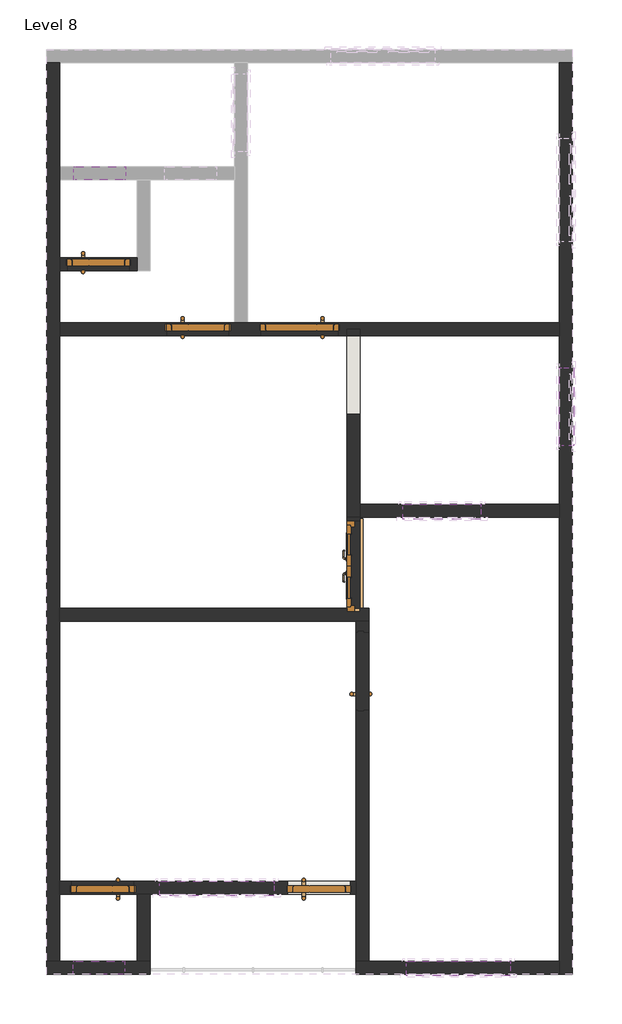
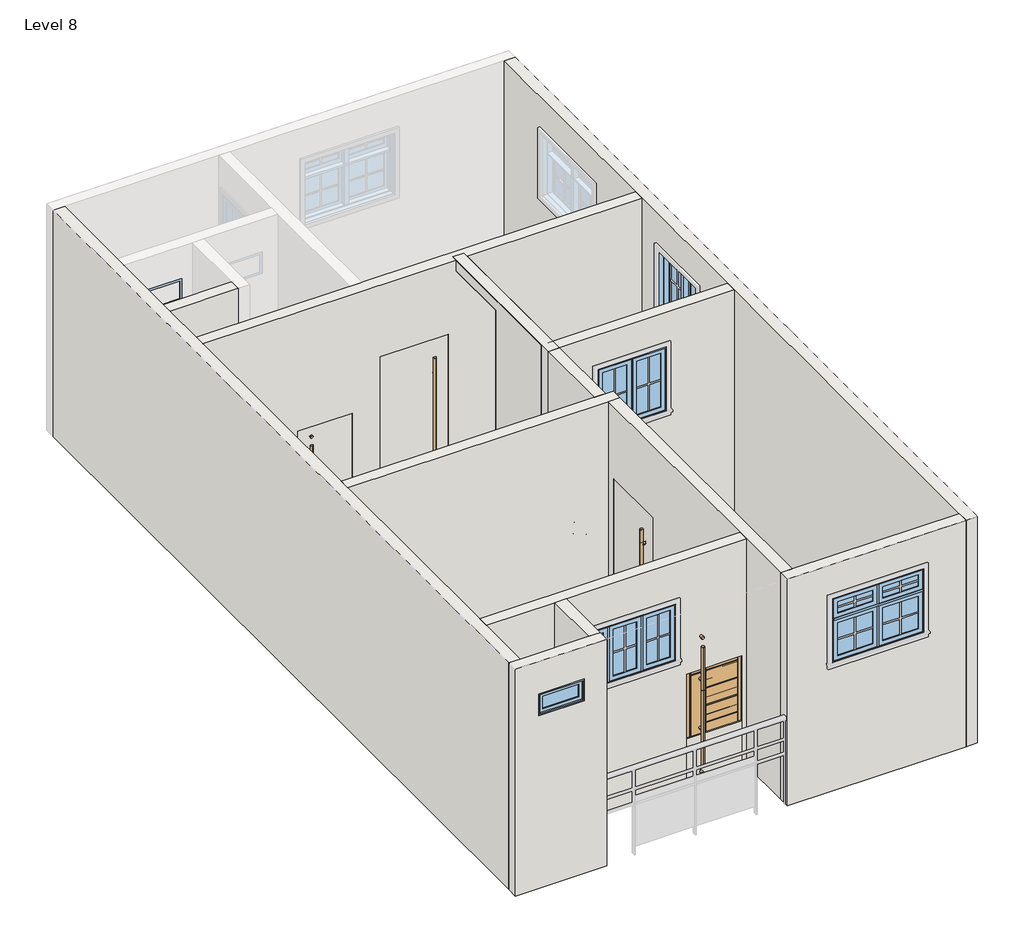
# One storey, part 1 of 2: 22 walls, 8 doors, 8 windows.
"""IFC4 building model written with IfcOpenShell, lengths in millimetres."""

from ifc_helpers import new_model, si_unit, frame, origin, place, context, project, spatial, polyline, outline, extrude, faceted_brep, transform, mapped, element, save
from components import door_9b787682, door_dc81b0c5, door_3_5c4206ef, door_3_79df91aa, door_2576ec39, door_55c03dfd, fixed_2_65c13adb, window_61697a4f, m_window_casement_double_3_e0bd8fa3, m_window_casement_double_awning_double_4_7efa9bbd

model = new_model("IFC4")

# Units and contexts
model_context = context("Model", 3, world=origin())
ifc_project = project(units=[si_unit("LENGTHUNIT", "METRE", prefix="MILLI")], contexts=[model_context])

# Site, building, storey
site = spatial("IfcSite", under=ifc_project)
building = spatial("IfcBuilding", under=site)
storey = spatial("IfcBuildingStorey", under=building, Name="Level 8", Elevation=13411.2)

# Doors
placement = place(None, origin())
door_shape = door_9b787682(model_context)
element("IfcDoor", 1, ObjectType="2'5\"", at=placement, inside=storey, context=model_context, shape_type="MappedRepresentation", body=[
    mapped(door_shape, transform((-22033.2963079, 3049.4742053, 13411.2), x_axis=(1.0, 0.0, 0.0), y_axis=(0.0, 1.0, 0.0), z_axis=(0.0, 0.0, 1.0))),
])
element("IfcDoor", 2, ObjectType="2'5\"", at=placement, inside=storey, context=model_context, shape_type="MappedRepresentation", body=[
    mapped(door_shape, transform((-23201.6963079, 3811.4742053, 13411.2), x_axis=(1.0, 0.0, 0.0), y_axis=(0.0, 1.0, 0.0), z_axis=(0.0, 0.0, 1.0))),
])
element("IfcDoor", 3, ObjectType="2'5\"", at=placement, inside=storey, context=model_context, shape_type="MappedRepresentation", body=[
    mapped(door_shape, transform((-23150.8963079, -3503.7257947, 13411.2), x_axis=(-1.0, 0.0, 0.0), y_axis=(0.0, -1.0, 0.0), z_axis=(0.0, 0.0, 1.0))),
])
door_2_shape = door_dc81b0c5(model_context)
element("IfcDoor", 4, ObjectType="2'5\"", at=placement, inside=storey, context=model_context, shape_type="MappedRepresentation", body=[
    mapped(door_2_shape, transform((-20610.8963079, -3503.7257947, 13457.4445349), x_axis=(1.0, 0.0, 0.0), y_axis=(0.0, 1.0, 0.0), z_axis=(0.0, 0.0, 1.0))),
])
element("IfcDoor", 5, ObjectType="2'5\"", at=placement, inside=storey, context=model_context, shape_type="MappedRepresentation", body=[
    mapped(door_2_shape, transform((-20610.8963079, -3503.7257947, 14067.0445349), x_axis=(1.0, 0.0, 0.0), y_axis=(0.0, 1.0, 0.0), z_axis=(0.0, 0.0, 1.0))),
])
door_3_shape = door_3_5c4206ef(model_context)
element("IfcDoor", 6, ObjectType="3'", at=placement, inside=storey, context=model_context, shape_type="MappedRepresentation", body=[
    mapped(door_3_shape, transform((-20102.8963079, -963.7257947, 13411.2), x_axis=(0.0, 1.0, 0.0), y_axis=(-1.0, 0.0, 0.0), z_axis=(0.0, 0.0, 1.0))),
])
door_3_2_shape = door_3_79df91aa(model_context)
element("IfcDoor", 7, ObjectType="3'", at=placement, inside=storey, context=model_context, shape_type="MappedRepresentation", body=[
    mapped(door_3_2_shape, transform((-20839.4963079, 3049.4742053, 13411.2), x_axis=(-1.0, 0.0, 0.0), y_axis=(0.0, -1.0, 0.0), z_axis=(0.0, 0.0, 1.0))),
])
door_4_shape = door_2576ec39(model_context)
door_5_shape = door_55c03dfd(model_context)
element("IfcDoor", 8, ObjectType="ExtDbl (8) : 3'6\"", at=placement, inside=storey, context=model_context, shape_type="MappedRepresentation", body=[
    mapped(door_4_shape, transform((-20204.4963079, 268.1742053, 13411.2), x_axis=(0.0, -1.0, 0.0), y_axis=(1.0, 0.0, 0.0), z_axis=(0.0, 0.0, 1.0))),
    mapped(door_5_shape, transform((-20204.4963079, 268.1742053, 13411.2), x_axis=(0.0, -1.0, 0.0), y_axis=(1.0, 0.0, 0.0), z_axis=(0.0, 0.0, 1.0))),
])

# Walls
element("IfcWall", 9, ObjectType="Generic - 6\"", at=placement, inside=storey, context=model_context, shape_type="Brep", body=[
    faceted_brep([(-17791.4963079, 6173.6742053, 13411.2), (-17791.4963079, 3125.6742053, 13411.2), (-17791.4963079, 2973.2742053, 13411.2), (-17791.4963079, 992.0742053, 13411.2), (-17791.4963079, 839.6742053, 13411.2), (-17791.4963079, -4367.3257947, 13411.2), (-17791.4963079, -4519.7257947, 13411.2), (-17791.4963079, -4519.7257947, 16611.6), (-17791.4963079, -4367.3257947, 16611.6), (-17791.4963079, 839.6742053, 16611.6), (-17791.4963079, 992.0742053, 16611.6), (-17791.4963079, 2973.2742053, 16611.6), (-17791.4963079, 3125.6742053, 16611.6), (-17791.4963079, 6173.6742053, 16611.6), (-17791.4963079, 4071.8242053, 16140.0), (-17791.4963079, 4071.8242053, 15240.0), (-17791.4963079, 5291.0242053, 15240.0), (-17791.4963079, 5291.0242053, 16140.0), (-17791.4963079, 1682.6367053, 16140.0), (-17791.4963079, 1682.6367053, 15240.0), (-17791.4963079, 2597.0367053, 15240.0), (-17791.4963079, 2597.0367053, 16140.0), (-17639.0963079, 6173.6742053, 13411.2), (-17639.0963079, 6173.6742053, 16611.6), (-17639.0963079, -4519.7257947, 16611.6), (-17639.0963079, -4519.7257947, 13411.2), (-17639.0963079, 4071.8242053, 16140.0), (-17639.0963079, 5291.0242053, 16140.0), (-17639.0963079, 5291.0242053, 15240.0), (-17639.0963079, 4071.8242053, 15240.0), (-17639.0963079, 1682.6367053, 16140.0), (-17639.0963079, 2597.0367053, 16140.0), (-17639.0963079, 2597.0367053, 15240.0), (-17639.0963079, 1682.6367053, 15240.0)], [[[0, 1, 2, 3, 4, 5, 6, 7, 8, 9, 10, 11, 12, 13], [14, 15, 16, 17], [18, 19, 20, 21]], [[22, 23, 24, 25], [26, 27, 28, 29], [30, 31, 32, 33]], [[6, 5, 4, 3, 2, 1, 0, 22, 25]], [[13, 12, 11, 10, 9, 8, 7, 24, 23]], [[0, 13, 23, 22]], [[7, 6, 25, 24]], [[15, 14, 26, 29]], [[16, 15, 29, 28]], [[17, 16, 28, 27]], [[14, 17, 27, 26]], [[19, 18, 30, 33]], [[20, 19, 33, 32]], [[21, 20, 32, 31]], [[18, 21, 31, 30]]]),
])
element("IfcWall", 10, ObjectType="Generic - 6\"", at=placement, inside=storey, context=model_context, shape_type="Brep", body=[
    faceted_brep([(-17791.4963079, -4367.3257947, 13411.2), (-20026.6963079, -4367.3257947, 13411.2), (-20179.0963079, -4367.3257947, 13411.2), (-20179.0963079, -4367.3257947, 16611.6), (-20026.6963079, -4367.3257947, 16611.6), (-17791.4963079, -4367.3257947, 16611.6), (-19585.5697454, -4367.3257947, 16140.0), (-19585.5697454, -4367.3257947, 15240.0), (-18366.3697454, -4367.3257947, 15240.0), (-18366.3697454, -4367.3257947, 16140.0), (-17791.4963079, -4519.7257947, 13411.2), (-17791.4963079, -4519.7257947, 16611.6), (-20179.0963079, -4519.7257947, 16611.6), (-20179.0963079, -4519.7257947, 13411.2), (-19585.5697454, -4519.7257947, 16140.0), (-18366.3697454, -4519.7257947, 16140.0), (-18366.3697454, -4519.7257947, 15240.0), (-19585.5697454, -4519.7257947, 15240.0)], [[[0, 1, 2, 3, 4, 5], [6, 7, 8, 9]], [[10, 11, 12, 13], [14, 15, 16, 17]], [[2, 1, 0, 10, 13]], [[5, 4, 3, 12, 11]], [[0, 5, 11, 10]], [[3, 2, 13, 12]], [[7, 6, 14, 17]], [[8, 7, 17, 16]], [[9, 8, 16, 15]], [[6, 9, 15, 14]]]),
])
element("IfcWall", 11, ObjectType="Generic - 6\"", at=placement, inside=storey, context=model_context, shape_type="Brep", body=[
    faceted_brep([(-23811.2963079, -4519.7257947, 13411.2), (-22592.0963079, -4519.7257947, 13411.2), (-22592.0963079, -4519.7257947, 16611.6), (-23811.2963079, -4519.7257947, 16611.6), (-23500.5431829, -4519.7257947, 16154.4), (-22890.9431829, -4519.7257947, 16154.4), (-22890.9431829, -4519.7257947, 15849.6), (-23500.5431829, -4519.7257947, 15849.6), (-23811.2963079, -4367.3257947, 13411.2), (-23811.2963079, -4367.3257947, 16611.6), (-23658.8963079, -4367.3257947, 16611.6), (-22744.4963079, -4367.3257947, 16611.6), (-22592.0963079, -4367.3257947, 16611.6), (-22592.0963079, -4367.3257947, 13411.2), (-22744.4963079, -4367.3257947, 13411.2), (-23658.8963079, -4367.3257947, 13411.2), (-23500.5431829, -4367.3257947, 16154.4), (-23500.5431829, -4367.3257947, 15849.6), (-22890.9431829, -4367.3257947, 15849.6), (-22890.9431829, -4367.3257947, 16154.4)], [[[0, 1, 2, 3], [4, 5, 6, 7]], [[8, 9, 10, 11, 12, 13, 14, 15], [16, 17, 18, 19]], [[1, 0, 8, 15, 14, 13]], [[3, 2, 12, 11, 10, 9]], [[0, 3, 9, 8]], [[2, 1, 13, 12]], [[17, 16, 4, 7]], [[18, 17, 7, 6]], [[19, 18, 6, 5]], [[16, 19, 5, 4]]]),
])
element("IfcWall", 12, ObjectType="Generic - 6\"", at=placement, inside=storey, context=model_context, shape_type="Brep", body=[
    faceted_brep([(-23658.8963079, -4367.3257947, 13411.2), (-23658.8963079, -3579.9257947, 13411.2), (-23658.8963079, -3427.5257947, 13411.2), (-23658.8963079, -379.5257947, 13411.2), (-23658.8963079, -227.1257947, 13411.2), (-23658.8963079, 2973.2742053, 13411.2), (-23658.8963079, 3125.6742053, 13411.2), (-23658.8963079, 3735.2742053, 13411.2), (-23658.8963079, 3887.6742053, 13411.2), (-23658.8963079, 4802.0742053, 13411.2), (-23658.8963079, 4954.4742053, 13411.2), (-23658.8963079, 6173.6742053, 13411.2), (-23658.8963079, 6173.6742053, 16611.6), (-23658.8963079, 4954.4742053, 16611.6), (-23658.8963079, 4802.0742053, 16611.6), (-23658.8963079, 3887.6742053, 16611.6), (-23658.8963079, 3735.2742053, 16611.6), (-23658.8963079, 3125.6742053, 16611.6), (-23658.8963079, 2973.2742053, 16611.6), (-23658.8963079, -227.1257947, 16611.6), (-23658.8963079, -379.5257947, 16611.6), (-23658.8963079, -3427.5257947, 16611.6), (-23658.8963079, -3579.9257947, 16611.6), (-23658.8963079, -4367.3257947, 16611.6), (-23811.2963079, -4367.3257947, 13411.2), (-23811.2963079, -4367.3257947, 16611.6), (-23811.2963079, 6173.6742053, 16611.6), (-23811.2963079, 6173.6742053, 13411.2)], [[[0, 1, 2, 3, 4, 5, 6, 7, 8, 9, 10, 11, 12, 13, 14, 15, 16, 17, 18, 19, 20, 21, 22, 23]], [[24, 25, 26, 27]], [[11, 10, 9, 8, 7, 6, 5, 4, 3, 2, 1, 0, 24, 27]], [[23, 22, 21, 20, 19, 18, 17, 16, 15, 14, 13, 12, 26, 25]], [[12, 11, 27, 26]], [[0, 23, 25, 24]]]),
])
element("IfcWall", 13, ObjectType="Generic - 6\"", at=placement, inside=storey, context=model_context, shape_type="Brep", body=[
    faceted_brep([(-17791.4963079, 2973.2742053, 16611.6), (-20128.2963079, 2973.2742053, 16611.6), (-20280.6963079, 2973.2742053, 16611.6), (-23658.8963079, 2973.2742053, 16611.6), (-23658.8963079, 2973.2742053, 13411.2), (-22401.5963079, 2973.2742053, 13411.2), (-22401.5963079, 2973.2742053, 14935.2), (-21664.9963079, 2973.2742053, 14935.2), (-21664.9963079, 2973.2742053, 13411.2), (-21296.6963079, 2973.2742053, 13411.2), (-21296.6963079, 2973.2742053, 15600.7), (-20382.2963079, 2973.2742053, 15600.7), (-20382.2963079, 2973.2742053, 13411.2), (-20280.6963079, 2973.2742053, 13411.2), (-20128.2963079, 2973.2742053, 13411.2), (-17791.4963079, 2973.2742053, 13411.2), (-23658.8963079, 3125.6742053, 16611.6), (-21601.4963079, 3125.6742053, 16611.6), (-21449.0963079, 3125.6742053, 16611.6), (-17791.4963079, 3125.6742053, 16611.6), (-17791.4963079, 3125.6742053, 13411.2), (-20382.2963079, 3125.6742053, 13411.2), (-20382.2963079, 3125.6742053, 15600.7), (-21296.6963079, 3125.6742053, 15600.7), (-21296.6963079, 3125.6742053, 13411.2), (-21449.0963079, 3125.6742053, 13411.2), (-21601.4963079, 3125.6742053, 13411.2), (-21664.9963079, 3125.6742053, 13411.2), (-21664.9963079, 3125.6742053, 14935.2), (-22401.5963079, 3125.6742053, 14935.2), (-22401.5963079, 3125.6742053, 13411.2), (-23658.8963079, 3125.6742053, 13411.2), (-22401.5963079, 3105.6742053, 13411.2), (-22416.5963079, 3105.6742053, 13411.2), (-22416.5963079, 3028.6742053, 13411.2), (-22401.5963079, 3028.6742053, 13411.2), (-20382.2963079, 3028.6742053, 13411.2), (-20367.2963079, 3028.6742053, 13411.2), (-20367.2963079, 3105.6742053, 13411.2), (-20382.2963079, 3105.6742053, 13411.2), (-21296.6963079, 3028.6742053, 13411.2), (-21664.9963079, 3028.6742053, 13411.2), (-21649.9963079, 3028.6742053, 13411.2), (-21649.9963079, 3105.6742053, 13411.2), (-21664.9963079, 3105.6742053, 13411.2), (-21296.6963079, 3105.6742053, 13411.2), (-21311.6963079, 3105.6742053, 13411.2), (-21311.6963079, 3028.6742053, 13411.2), (-21296.6963079, 3105.6742053, 15600.7), (-20382.2963079, 3105.6742053, 15600.7), (-20382.2963079, 3028.6742053, 15600.7), (-21296.6963079, 3028.6742053, 15600.7), (-21311.6963079, 3105.6742053, 15615.7), (-20367.2963079, 3105.6742053, 15615.7), (-20367.2963079, 3028.6742053, 15615.7), (-21311.6963079, 3028.6742053, 15615.7), (-21664.9963079, 3105.6742053, 14935.2), (-22401.5963079, 3105.6742053, 14935.2), (-22401.5963079, 3028.6742053, 14935.2), (-21664.9963079, 3028.6742053, 14935.2), (-22416.5963079, 3105.6742053, 14950.2), (-21649.9963079, 3105.6742053, 14950.2), (-21649.9963079, 3028.6742053, 14950.2), (-22416.5963079, 3028.6742053, 14950.2)], [[[0, 1, 2, 3, 4, 5, 6, 7, 8, 9, 10, 11, 12, 13, 14, 15]], [[16, 17, 18, 19, 20, 21, 22, 23, 24, 25, 26, 27, 28, 29, 30, 31]], [[4, 31, 30, 32, 33, 34, 35, 5]], [[20, 15, 14, 13, 12, 36, 37, 38, 39, 21]], [[40, 9, 8, 41, 42, 43, 44, 27, 26, 25, 24, 45, 46, 47]], [[3, 2, 1, 0, 19, 18, 17, 16]], [[0, 15, 20, 19]], [[4, 3, 16, 31]], [[48, 23, 22, 49]], [[50, 11, 10, 51]], [[23, 48, 45, 24]], [[51, 10, 9, 40]], [[49, 22, 21, 39]], [[11, 50, 36, 12]], [[52, 53, 54, 55]], [[52, 55, 47, 46]], [[50, 51, 40, 47, 55, 54, 37, 36]], [[54, 53, 38, 37]], [[48, 49, 39, 38, 53, 52, 46, 45]], [[28, 56, 57, 29]], [[6, 58, 59, 7]], [[56, 28, 27, 44]], [[7, 59, 41, 8]], [[29, 57, 32, 30]], [[58, 6, 5, 35]], [[60, 61, 62, 63]], [[62, 61, 43, 42]], [[59, 58, 35, 34, 63, 62, 42, 41]], [[60, 63, 34, 33]], [[57, 56, 44, 43, 61, 60, 33, 32]]]),
])
element("IfcWall", 14, ObjectType="Generic - 6\"", at=placement, inside=storey, context=model_context, shape_type="Brep", body=[
    faceted_brep([(-20280.6963079, 3049.4742053, 16611.6), (-20280.6963079, 3049.4742053, 13411.2), (-20280.6963079, 839.6742053, 13411.2), (-20280.6963079, 839.6742053, 16611.6), (-20280.6963079, 2974.7724011, 16459.2), (-20280.6963079, 2050.5574639, 16459.2), (-20280.6963079, 2050.5574639, 14020.8), (-20280.6963079, 2974.7724011, 14020.8), (-20128.2963079, 839.6742053, 13411.2), (-20128.2963079, 992.0742053, 13411.2), (-20128.2963079, 3049.4742053, 13411.2), (-20128.2963079, 3049.4742053, 16611.6), (-20128.2963079, 992.0742053, 16611.6), (-20128.2963079, 839.6742053, 16611.6), (-20128.2963079, 2050.5574639, 16459.2), (-20128.2963079, 2974.7724011, 16459.2), (-20128.2963079, 2974.7724011, 14020.8), (-20128.2963079, 2050.5574639, 14020.8)], [[[0, 1, 2, 3], [4, 5, 6, 7]], [[8, 9, 10, 11, 12, 13], [14, 15, 16, 17]], [[2, 1, 10, 9, 8]], [[0, 3, 13, 12, 11]], [[3, 2, 8, 13]], [[4, 15, 14, 5]], [[6, 17, 16, 7]], [[15, 4, 7, 16]], [[5, 14, 17, 6]], [[0, 11, 10, 1]]]),
])
element("IfcWall", 15, ObjectType="Generic - 6\"", at=placement, inside=storey, context=model_context, shape_type="SweptSolid", body=[
    extrude(outline(polyline([(13411.2, -20128.2963079), (13411.2, -17791.4963079), (16611.6, -17791.4963079), (16611.6, -20128.2963079), (13411.2, -20128.2963079)]), holes=[polyline([(16140.0, -19624.1658391), (16140.0, -18709.7658391), (15240.0, -18709.7658391), (15240.0, -19624.1658391), (16140.0, -19624.1658391)])]), frame((0.0, 839.6742053, 0.0), z_axis=(0.0, 1.0, 0.0), x_axis=(0.0, 0.0, 1.0)), (0.0, 0.0, 1.0), 152.4),
])
element("IfcWall", 16, ObjectType="Generic - 6\"", at=placement, inside=storey, context=model_context, shape_type="Brep", body=[
    faceted_brep([(-23658.8963079, -379.5257947, 13411.2), (-20179.0963079, -379.5257947, 13411.2), (-20026.6963079, -379.5257947, 13411.2), (-20026.6963079, -379.5257947, 16611.6), (-20179.0963079, -379.5257947, 16611.6), (-23658.8963079, -379.5257947, 16611.6), (-23658.8963079, -227.1257947, 16611.6), (-20280.6963079, -227.1257947, 16611.6), (-20128.2963079, -227.1257947, 16611.6), (-20026.6963079, -227.1257947, 16611.6), (-20026.6963079, -227.1257947, 13411.2), (-20128.2963079, -227.1257947, 13411.2), (-20128.2963079, -227.1257947, 15521.2), (-20280.6963079, -227.1257947, 15521.2), (-20280.6963079, -227.1257947, 13411.2), (-23658.8963079, -227.1257947, 13411.2), (-20280.6963079, -265.2257947, 13411.2), (-20128.2963079, -265.2257947, 13411.2), (-20280.6963079, -265.2257947, 15521.2), (-20128.2963079, -265.2257947, 15521.2)], [[[0, 1, 2, 3, 4, 5]], [[6, 7, 8, 9, 10, 11, 12, 13, 14, 15]], [[2, 1, 0, 15, 14, 16, 17, 11, 10]], [[5, 4, 3, 9, 8, 7, 6]], [[0, 5, 6, 15]], [[3, 2, 10, 9]], [[18, 16, 14, 13]], [[17, 19, 12, 11]], [[19, 18, 13, 12]], [[16, 18, 19, 17]]]),
])
element("IfcWall", 17, ObjectType="Generic - 6\"", at=placement, inside=storey, context=model_context, shape_type="Brep", body=[
    faceted_brep([(-20179.0963079, -4367.3257947, 16611.6), (-20179.0963079, -3579.9257947, 16611.6), (-20179.0963079, -3427.5257947, 16611.6), (-20179.0963079, -379.5257947, 16611.6), (-20179.0963079, -379.5257947, 13411.2), (-20179.0963079, -506.5257947, 13411.2), (-20179.0963079, -506.5257947, 15600.7), (-20179.0963079, -1420.9257947, 15600.7), (-20179.0963079, -1420.9257947, 13411.2), (-20179.0963079, -3427.5257947, 13411.2), (-20179.0963079, -3579.9257947, 13411.2), (-20179.0963079, -4367.3257947, 13411.2), (-20026.6963079, -379.5257947, 16611.6), (-20026.6963079, -4367.3257947, 16611.6), (-20026.6963079, -4367.3257947, 13411.2), (-20026.6963079, -1420.9257947, 13411.2), (-20026.6963079, -1420.9257947, 15600.7), (-20026.6963079, -506.5257947, 15600.7), (-20026.6963079, -506.5257947, 13411.2), (-20026.6963079, -379.5257947, 13411.2), (-20082.0963079, -506.5257947, 13411.2), (-20082.0963079, -491.5257947, 13411.2), (-20159.0963079, -491.5257947, 13411.2), (-20159.0963079, -506.5257947, 13411.2), (-20159.0963079, -1420.9257947, 13411.2), (-20159.0963079, -1435.9257947, 13411.2), (-20082.0963079, -1435.9257947, 13411.2), (-20082.0963079, -1420.9257947, 13411.2), (-20159.0963079, -506.5257947, 15600.7), (-20159.0963079, -1420.9257947, 15600.7), (-20082.0963079, -1420.9257947, 15600.7), (-20082.0963079, -506.5257947, 15600.7), (-20159.0963079, -1435.9257947, 15615.7), (-20159.0963079, -491.5257947, 15615.7), (-20082.0963079, -491.5257947, 15615.7), (-20082.0963079, -1435.9257947, 15615.7)], [[[0, 1, 2, 3, 4, 5, 6, 7, 8, 9, 10, 11]], [[12, 13, 14, 15, 16, 17, 18, 19]], [[4, 19, 18, 20, 21, 22, 23, 5]], [[14, 11, 10, 9, 8, 24, 25, 26, 27, 15]], [[3, 2, 1, 0, 13, 12]], [[0, 11, 14, 13]], [[4, 3, 12, 19]], [[6, 28, 29, 7]], [[16, 30, 31, 17]], [[28, 6, 5, 23]], [[17, 31, 20, 18]], [[7, 29, 24, 8]], [[30, 16, 15, 27]], [[32, 33, 34, 35]], [[34, 33, 22, 21]], [[31, 30, 27, 26, 35, 34, 21, 20]], [[32, 35, 26, 25]], [[29, 28, 23, 22, 33, 32, 25, 24]]]),
])
element("IfcWall", 18, ObjectType="Generic - 6\"", at=placement, inside=storey, context=model_context, shape_type="Brep", body=[
    faceted_brep([(-20179.0963079, -3579.9257947, 16611.6), (-22592.0963079, -3579.9257947, 16611.6), (-22744.4963079, -3579.9257947, 16611.6), (-23658.8963079, -3579.9257947, 16611.6), (-23658.8963079, -3579.9257947, 13411.2), (-23519.1963079, -3579.9257947, 13411.2), (-23519.1963079, -3579.9257947, 14935.2), (-22782.5963079, -3579.9257947, 14935.2), (-22782.5963079, -3579.9257947, 13411.2), (-22744.4963079, -3579.9257947, 13411.2), (-22592.0963079, -3579.9257947, 13411.2), (-20179.0963079, -3579.9257947, 13411.2), (-22484.1463079, -3579.9257947, 15240.0), (-22484.1463079, -3579.9257947, 16040.0), (-21137.9463079, -3579.9257947, 16040.0), (-21137.9463079, -3579.9257947, 15240.0), (-20979.1963079, -3579.9257947, 14981.4445349), (-20242.5963079, -3579.9257947, 14981.4445349), (-20242.5963079, -3579.9257947, 13457.4445349), (-20979.1963079, -3579.9257947, 13457.4445349), (-23658.8963079, -3427.5257947, 16611.6), (-20179.0963079, -3427.5257947, 16611.6), (-20179.0963079, -3427.5257947, 13411.2), (-22782.5963079, -3427.5257947, 13411.2), (-22782.5963079, -3427.5257947, 14935.2), (-23519.1963079, -3427.5257947, 14935.2), (-23519.1963079, -3427.5257947, 13411.2), (-23658.8963079, -3427.5257947, 13411.2), (-22484.1463079, -3427.5257947, 16040.0), (-22484.1463079, -3427.5257947, 15240.0), (-21137.9463079, -3427.5257947, 15240.0), (-21137.9463079, -3427.5257947, 16040.0), (-20242.5963079, -3427.5257947, 14981.4445349), (-20979.1963079, -3427.5257947, 14981.4445349), (-20979.1963079, -3427.5257947, 13457.4445349), (-20242.5963079, -3427.5257947, 13457.4445349), (-23519.1963079, -3482.9257947, 13411.2), (-23534.1963079, -3482.9257947, 13411.2), (-23534.1963079, -3559.9257947, 13411.2), (-23519.1963079, -3559.9257947, 13411.2), (-22782.5963079, -3559.9257947, 13411.2), (-22767.5963079, -3559.9257947, 13411.2), (-22767.5963079, -3482.9257947, 13411.2), (-22782.5963079, -3482.9257947, 13411.2), (-20979.1963079, -3559.9257947, 14981.4445349), (-20242.5963079, -3559.9257947, 14981.4445349), (-20242.5963079, -3482.9257947, 14981.4445349), (-20979.1963079, -3482.9257947, 14981.4445349), (-20242.5963079, -3559.9257947, 13457.4445349), (-20242.5963079, -3482.9257947, 13457.4445349), (-20227.5963079, -3559.9257947, 13457.4445349), (-20227.5963079, -3482.9257947, 13457.4445349), (-20979.1963079, -3482.9257947, 13457.4445349), (-20994.1963079, -3482.9257947, 13457.4445349), (-20994.1963079, -3559.9257947, 13457.4445349), (-20979.1963079, -3559.9257947, 13457.4445349), (-20994.1963079, -3559.9257947, 14996.4445349), (-20994.1963079, -3482.9257947, 14996.4445349), (-20227.5963079, -3482.9257947, 14996.4445349), (-20227.5963079, -3559.9257947, 14996.4445349), (-23519.1963079, -3559.9257947, 14935.2), (-22782.5963079, -3559.9257947, 14935.2), (-22782.5963079, -3482.9257947, 14935.2), (-23519.1963079, -3482.9257947, 14935.2), (-22767.5963079, -3559.9257947, 14950.2), (-23534.1963079, -3559.9257947, 14950.2), (-23534.1963079, -3482.9257947, 14950.2), (-22767.5963079, -3482.9257947, 14950.2)], [[[0, 1, 2, 3, 4, 5, 6, 7, 8, 9, 10, 11], [12, 13, 14, 15], [16, 17, 18, 19]], [[20, 21, 22, 23, 24, 25, 26, 27], [28, 29, 30, 31], [32, 33, 34, 35]], [[4, 27, 26, 36, 37, 38, 39, 5]], [[22, 11, 10, 9, 8, 40, 41, 42, 43, 23]], [[3, 2, 1, 0, 21, 20]], [[4, 3, 20, 27]], [[0, 11, 22, 21]], [[29, 28, 13, 12]], [[30, 29, 12, 15]], [[31, 30, 15, 14]], [[28, 31, 14, 13]], [[16, 44, 45, 17]], [[32, 46, 47, 33]], [[17, 45, 48, 18]], [[46, 32, 35, 49]], [[18, 48, 50, 51, 49, 35, 34, 52, 53, 54, 55, 19]], [[44, 16, 19, 55]], [[33, 47, 52, 34]], [[56, 57, 58, 59]], [[51, 50, 59, 58]], [[47, 46, 49, 51, 58, 57, 53, 52]], [[54, 53, 57, 56]], [[45, 44, 55, 54, 56, 59, 50, 48]], [[6, 60, 61, 7]], [[24, 62, 63, 25]], [[60, 6, 5, 39]], [[25, 63, 36, 26]], [[7, 61, 40, 8]], [[62, 24, 23, 43]], [[64, 65, 66, 67]], [[66, 65, 38, 37]], [[63, 62, 43, 42, 67, 66, 37, 36]], [[64, 67, 42, 41]], [[61, 60, 39, 38, 65, 64, 41, 40]]]),
])
element("IfcWall", 19, ObjectType="Generic - 6\"", at=placement, inside=storey, context=model_context, shape_type="SweptSolid", body=[
    extrude(outline(polyline([(-22744.4963079, -4367.3257947), (-22744.4963079, -3579.9257947), (-22592.0963079, -3579.9257947), (-22592.0963079, -4367.3257947), (-22744.4963079, -4367.3257947)])), frame((0.0, 0.0, 13411.2), z_axis=(0.0, 0.0, 1.0), x_axis=(1.0, 0.0, 0.0)), (0.0, 0.0, 1.0), 3200.4),
])
element("IfcWall", 20, ObjectType="Generic - 6\"", at=placement, inside=storey, context=model_context, shape_type="Brep", body=[
    faceted_brep([(-22744.4963079, 3735.2742053, 16611.6), (-23658.8963079, 3735.2742053, 16611.6), (-23658.8963079, 3735.2742053, 13411.2), (-23569.9963079, 3735.2742053, 13411.2), (-23569.9963079, 3735.2742053, 14935.2), (-22833.3963079, 3735.2742053, 14935.2), (-22833.3963079, 3735.2742053, 13411.2), (-22744.4963079, 3735.2742053, 13411.2), (-23658.8963079, 3887.6742053, 16611.6), (-22744.4963079, 3887.6742053, 16611.6), (-22744.4963079, 3887.6742053, 13411.2), (-22833.3963079, 3887.6742053, 13411.2), (-22833.3963079, 3887.6742053, 14935.2), (-23569.9963079, 3887.6742053, 14935.2), (-23569.9963079, 3887.6742053, 13411.2), (-23658.8963079, 3887.6742053, 13411.2), (-23569.9963079, 3867.6742053, 13411.2), (-23584.9963079, 3867.6742053, 13411.2), (-23584.9963079, 3790.6742053, 13411.2), (-23569.9963079, 3790.6742053, 13411.2), (-22833.3963079, 3790.6742053, 13411.2), (-22818.3963079, 3790.6742053, 13411.2), (-22818.3963079, 3867.6742053, 13411.2), (-22833.3963079, 3867.6742053, 13411.2), (-22833.3963079, 3867.6742053, 14935.2), (-23569.9963079, 3867.6742053, 14935.2), (-23569.9963079, 3790.6742053, 14935.2), (-22833.3963079, 3790.6742053, 14935.2), (-23584.9963079, 3867.6742053, 14950.2), (-22818.3963079, 3867.6742053, 14950.2), (-22818.3963079, 3790.6742053, 14950.2), (-23584.9963079, 3790.6742053, 14950.2)], [[[0, 1, 2, 3, 4, 5, 6, 7]], [[8, 9, 10, 11, 12, 13, 14, 15]], [[2, 15, 14, 16, 17, 18, 19, 3]], [[10, 7, 6, 20, 21, 22, 23, 11]], [[1, 0, 9, 8]], [[0, 7, 10, 9]], [[2, 1, 8, 15]], [[12, 24, 25, 13]], [[4, 26, 27, 5]], [[24, 12, 11, 23]], [[5, 27, 20, 6]], [[13, 25, 16, 14]], [[26, 4, 3, 19]], [[28, 29, 30, 31]], [[30, 29, 22, 21]], [[27, 26, 19, 18, 31, 30, 21, 20]], [[28, 31, 18, 17]], [[25, 24, 23, 22, 29, 28, 17, 16]]]),
])
element("IfcWall", 21, ObjectType="Generic - 6\"", at=placement, inside=storey, context=model_context, shape_type="Brep", body=[
    faceted_brep([(-20280.6963079, -227.1257947, 16611.6), (-20280.6963079, 839.6742053, 16611.6), (-20280.6963079, 839.6742053, 13411.2), (-20280.6963079, 801.5742053, 13411.2), (-20280.6963079, 801.5742053, 15521.2), (-20280.6963079, -227.1257947, 15521.2), (-20128.2963079, 839.6742053, 16611.6), (-20128.2963079, -227.1257947, 16611.6), (-20128.2963079, -227.1257947, 15521.2), (-20128.2963079, 801.5742053, 15521.2), (-20128.2963079, 801.5742053, 13411.2), (-20128.2963079, 839.6742053, 13411.2), (-20179.0963079, -227.1257947, 16611.6), (-20179.0963079, -227.1257947, 15521.2)], [[[0, 1, 2, 3, 4, 5]], [[6, 7, 8, 9, 10, 11]], [[2, 11, 10, 3]], [[1, 0, 12, 7, 6]], [[2, 1, 6, 11]], [[7, 12, 0, 5, 13, 8]], [[4, 9, 8, 13, 5]], [[9, 4, 3, 10]]]),
])
element("IfcWall", 22, ObjectType="Generic - 6\"", at=placement, inside=storey, context=model_context, shape_type="Brep", body=[
    faceted_brep([(-23658.8963079, 2973.2742053, 13411.2), (-20280.6963079, 2973.2742053, 13411.2), (-20128.2963079, 2973.2742053, 13411.2), (-17791.4963079, 2973.2742053, 13411.2), (-17791.4963079, 2973.2742053, 16611.6), (-20128.2963079, 2973.2742053, 16611.6), (-20280.6963079, 2973.2742053, 16611.6), (-23658.8963079, 2973.2742053, 16611.6), (-23658.8963079, 3125.6742053, 13411.2), (-23658.8963079, 3125.6742053, 16611.6), (-21601.4963079, 3125.6742053, 16611.6), (-21449.0963079, 3125.6742053, 16611.6), (-17791.4963079, 3125.6742053, 16611.6), (-17791.4963079, 3125.6742053, 13411.2), (-21449.0963079, 3125.6742053, 13411.2), (-21601.4963079, 3125.6742053, 13411.2)], [[[0, 1, 2, 3, 4, 5, 6, 7]], [[8, 9, 10, 11, 12, 13, 14, 15]], [[3, 2, 1, 0, 8, 15, 14, 13]], [[7, 6, 5, 4, 12, 11, 10, 9]], [[0, 7, 9, 8]], [[4, 3, 13, 12]]]),
])
element("IfcWall", 23, ObjectType="Generic - 6\"", at=placement, inside=storey, context=model_context, shape_type="SweptSolid", body=[
    extrude(outline(polyline([(2973.2742053, 13411.2), (992.0742053, 13411.2), (992.0742053, 16611.6), (2973.2742053, 16611.6), (2973.2742053, 16459.2), (2050.5574639, 16459.2), (2050.5574639, 14020.8), (2973.2742053, 14020.8), (2973.2742053, 13411.2)])), frame((-20280.6963079, 0.0, 0.0), z_axis=(1.0, 0.0, 0.0), x_axis=(0.0, 1.0, 0.0)), (0.0, 0.0, 1.0), 152.4),
])
element("IfcWall", 24, ObjectType="Generic - 6\"", at=placement, inside=storey, context=model_context, shape_type="SweptSolid", body=[
    extrude(outline(polyline([(13411.2, -20128.2963079), (13411.2, -17791.4963079), (16611.6, -17791.4963079), (16611.6, -20128.2963079), (13411.2, -20128.2963079)]), holes=[polyline([(16140.0, -19624.1658391), (16140.0, -18709.7658391), (15240.0, -18709.7658391), (15240.0, -19624.1658391), (16140.0, -19624.1658391)])]), frame((0.0, 839.6742053, 0.0), z_axis=(0.0, 1.0, 0.0), x_axis=(0.0, 0.0, 1.0)), (0.0, 0.0, 1.0), 152.4),
])
element("IfcWall", 25, ObjectType="Generic - 6\"", at=placement, inside=storey, context=model_context, shape_type="Brep", body=[
    faceted_brep([(-23658.8963079, -379.5257947, 13411.2), (-20179.0963079, -379.5257947, 13411.2), (-20179.0963079, -379.5257947, 16611.6), (-23658.8963079, -379.5257947, 16611.6), (-23658.8963079, -227.1257947, 16611.6), (-20280.6963079, -227.1257947, 16611.6), (-20179.0963079, -227.1257947, 16611.6), (-20179.0963079, -227.1257947, 15521.2), (-20280.6963079, -227.1257947, 15521.2), (-20280.6963079, -227.1257947, 13411.2), (-23658.8963079, -227.1257947, 13411.2), (-20280.6963079, -265.2257947, 13411.2), (-20179.0963079, -265.2257947, 13411.2), (-20179.0963079, -265.2257947, 15521.2), (-20280.6963079, -265.2257947, 15521.2)], [[[0, 1, 2, 3]], [[4, 5, 6, 7, 8, 9, 10]], [[1, 0, 10, 9, 11, 12]], [[3, 2, 6, 5, 4]], [[2, 1, 12, 13, 7, 6]], [[14, 11, 9, 8]], [[11, 14, 13, 12]], [[14, 8, 7, 13]], [[0, 3, 4, 10]]]),
])
element("IfcWall", 26, ObjectType="Generic - 6\"", at=placement, inside=storey, context=model_context, shape_type="Brep", body=[
    faceted_brep([(-20179.0963079, -379.5257947, 13411.2), (-20179.0963079, -3427.5257947, 13411.2), (-20179.0963079, -3579.9257947, 13411.2), (-20179.0963079, -4367.3257947, 13411.2), (-20179.0963079, -4367.3257947, 16611.6), (-20179.0963079, -3579.9257947, 16611.6), (-20179.0963079, -3427.5257947, 16611.6), (-20179.0963079, -379.5257947, 16611.6), (-20026.6963079, -379.5257947, 13411.2), (-20026.6963079, -379.5257947, 16611.6), (-20026.6963079, -4367.3257947, 16611.6), (-20026.6963079, -4367.3257947, 13411.2)], [[[0, 1, 2, 3, 4, 5, 6, 7]], [[8, 9, 10, 11]], [[3, 2, 1, 0, 8, 11]], [[7, 6, 5, 4, 10, 9]], [[4, 3, 11, 10]], [[0, 7, 9, 8]]]),
])
element("IfcWall", 27, ObjectType="Generic - 6\"", at=placement, inside=storey, context=model_context, shape_type="Brep", body=[
    faceted_brep([(-23658.8963079, -3579.9257947, 13411.2), (-22744.4963079, -3579.9257947, 13411.2), (-22592.0963079, -3579.9257947, 13411.2), (-20179.0963079, -3579.9257947, 13411.2), (-20179.0963079, -3579.9257947, 16611.6), (-22592.0963079, -3579.9257947, 16611.6), (-22744.4963079, -3579.9257947, 16611.6), (-23658.8963079, -3579.9257947, 16611.6), (-22484.1463079, -3579.9257947, 15240.0), (-22484.1463079, -3579.9257947, 16040.0), (-21137.9463079, -3579.9257947, 16040.0), (-21137.9463079, -3579.9257947, 15240.0), (-20979.1963079, -3579.9257947, 15591.0445349), (-20242.5963079, -3579.9257947, 15591.0445349), (-20242.5963079, -3579.9257947, 14067.0445349), (-20979.1963079, -3579.9257947, 14067.0445349), (-20179.0963079, -3427.5257947, 13411.2), (-23658.8963079, -3427.5257947, 13411.2), (-23658.8963079, -3427.5257947, 16611.6), (-20179.0963079, -3427.5257947, 16611.6), (-22484.1463079, -3427.5257947, 16040.0), (-22484.1463079, -3427.5257947, 15240.0), (-21137.9463079, -3427.5257947, 15240.0), (-21137.9463079, -3427.5257947, 16040.0), (-20242.5963079, -3427.5257947, 15591.0445349), (-20979.1963079, -3427.5257947, 15591.0445349), (-20979.1963079, -3427.5257947, 14067.0445349), (-20242.5963079, -3427.5257947, 14067.0445349), (-20979.1963079, -3559.9257947, 15591.0445349), (-20242.5963079, -3559.9257947, 15591.0445349), (-20242.5963079, -3482.9257947, 15591.0445349), (-20979.1963079, -3482.9257947, 15591.0445349), (-20242.5963079, -3559.9257947, 14067.0445349), (-20242.5963079, -3482.9257947, 14067.0445349), (-20227.5963079, -3559.9257947, 14067.0445349), (-20227.5963079, -3482.9257947, 14067.0445349), (-20979.1963079, -3482.9257947, 14067.0445349), (-20994.1963079, -3482.9257947, 14067.0445349), (-20994.1963079, -3559.9257947, 14067.0445349), (-20979.1963079, -3559.9257947, 14067.0445349), (-20994.1963079, -3559.9257947, 15606.0445349), (-20994.1963079, -3482.9257947, 15606.0445349), (-20227.5963079, -3482.9257947, 15606.0445349), (-20227.5963079, -3559.9257947, 15606.0445349)], [[[0, 1, 2, 3, 4, 5, 6, 7], [8, 9, 10, 11], [12, 13, 14, 15]], [[16, 17, 18, 19], [20, 21, 22, 23], [24, 25, 26, 27]], [[3, 2, 1, 0, 17, 16]], [[7, 6, 5, 4, 19, 18]], [[4, 3, 16, 19]], [[21, 20, 9, 8]], [[22, 21, 8, 11]], [[23, 22, 11, 10]], [[20, 23, 10, 9]], [[12, 28, 29, 13]], [[24, 30, 31, 25]], [[13, 29, 32, 14]], [[30, 24, 27, 33]], [[14, 32, 34, 35, 33, 27, 26, 36, 37, 38, 39, 15]], [[28, 12, 15, 39]], [[25, 31, 36, 26]], [[40, 41, 42, 43]], [[35, 34, 43, 42]], [[31, 30, 33, 35, 42, 41, 37, 36]], [[38, 37, 41, 40]], [[29, 28, 39, 38, 40, 43, 34, 32]], [[0, 7, 18, 17]]]),
])
element("IfcWall", 28, ObjectType="Generic - 6\"", at=placement, inside=storey, context=model_context, shape_type="SweptSolid", body=[
    extrude(outline(polyline([(-22744.4963079, -4367.3257947), (-22744.4963079, -3579.9257947), (-22592.0963079, -3579.9257947), (-22592.0963079, -4367.3257947), (-22744.4963079, -4367.3257947)])), frame((0.0, 0.0, 13411.2), z_axis=(0.0, 0.0, 1.0), x_axis=(1.0, 0.0, 0.0)), (0.0, 0.0, 1.0), 3200.4),
])
element("IfcWall", 29, ObjectType="Generic - 6\"", at=placement, inside=storey, context=model_context, shape_type="SweptSolid", body=[
    extrude(outline(polyline([(-22744.4963079, 3735.2742053), (-23658.8963079, 3735.2742053), (-23658.8963079, 3887.6742053), (-22744.4963079, 3887.6742053), (-22744.4963079, 3735.2742053)])), frame((0.0, 0.0, 13411.2), z_axis=(0.0, 0.0, 1.0), x_axis=(1.0, 0.0, 0.0)), (0.0, 0.0, 1.0), 3200.4),
])
element("IfcWall", 30, ObjectType="Generic - 6\"", at=placement, inside=storey, context=model_context, shape_type="Brep", body=[
    faceted_brep([(-20280.6963079, 839.6742053, 13411.2), (-20280.6963079, -227.1257947, 13411.2), (-20280.6963079, -227.1257947, 16611.6), (-20280.6963079, 839.6742053, 16611.6), (-20128.2963079, 839.6742053, 13411.2), (-20128.2963079, 839.6742053, 16611.6), (-20128.2963079, -227.1257947, 16611.6), (-20128.2963079, -227.1257947, 13411.2), (-20179.0963079, -227.1257947, 16611.6)], [[[0, 1, 2, 3]], [[4, 5, 6, 7]], [[1, 0, 4, 7]], [[3, 2, 8, 6, 5]], [[2, 1, 7, 6, 8]], [[0, 3, 5, 4]]]),
])

# Windows
fixed_2_shape = fixed_2_65c13adb(model_context)
element("IfcWindow", 31, ObjectType="Fixed : 2'", at=placement, inside=storey, context=model_context, shape_type="MappedRepresentation", body=[
    mapped(fixed_2_shape, transform((-23233.8431829, -4443.5257947, 14935.2), x_axis=(-1.0, 0.0, 0.0), y_axis=(0.0, -1.0, 0.0), z_axis=(0.0, 0.0, 1.0))),
])
element("IfcWindow", 32, ObjectType="Fixed : 2'", at=placement, inside=storey, context=model_context, shape_type="MappedRepresentation", body=[
    mapped(fixed_2_shape, transform((-23147.2252141, 4878.2742053, 14935.2), x_axis=(1.0, 0.0, 0.0), y_axis=(0.0, 1.0, 0.0), z_axis=(0.0, 0.0, 1.0))),
])
window_shape = window_61697a4f(model_context)
element("IfcWindow", 33, ObjectType="M_Window-Awning-Triple-Horizontal : 4'5\"", at=placement, inside=storey, context=model_context, shape_type="MappedRepresentation", body=[
    mapped(window_shape, transform((-21811.0463079, -3503.7257947, 14340.0), x_axis=(-1.0, 0.0, 0.0), y_axis=(0.0, -1.0, 0.0), z_axis=(0.0, 0.0, 1.0))),
])
element("IfcWindow", 34, ObjectType="M_Window-Awning-Triple-Horizontal : 4'5\"", at=placement, inside=storey, context=model_context, shape_type="MappedRepresentation", body=[
    mapped(window_shape, transform((-21811.0463079, -3503.7257947, 14340.0), x_axis=(-1.0, 0.0, 0.0), y_axis=(0.0, -1.0, 0.0), z_axis=(0.0, 0.0, 1.0))),
])
m_window_casement_double_3_shape = m_window_casement_double_3_e0bd8fa3(model_context)
element("IfcWindow", 35, ObjectType="M_Window-Casement-Double : 3'", at=placement, inside=storey, context=model_context, shape_type="MappedRepresentation", body=[
    mapped(m_window_casement_double_3_shape, transform((-19166.9658391, 915.8742053, 14340.0), x_axis=(-1.0, 0.0, 0.0), y_axis=(0.0, -1.0, 0.0), z_axis=(0.0, 0.0, 1.0))),
])
element("IfcWindow", 36, ObjectType="M_Window-Casement-Double : 3'", at=placement, inside=storey, context=model_context, shape_type="MappedRepresentation", body=[
    mapped(m_window_casement_double_3_shape, transform((-17715.2963079, 2139.8367053, 14340.0), x_axis=(0.0, -1.0, 0.0), y_axis=(1.0, 0.0, 0.0), z_axis=(0.0, 0.0, 1.0))),
])
element("IfcWindow", 37, ObjectType="M_Window-Casement-Double : 3'", at=placement, inside=storey, context=model_context, shape_type="MappedRepresentation", body=[
    mapped(m_window_casement_double_3_shape, transform((-19166.9658391, 915.8742053, 14340.0), x_axis=(-1.0, 0.0, 0.0), y_axis=(0.0, -1.0, 0.0), z_axis=(0.0, 0.0, 1.0))),
])
m_window_casement_double_awning_double_4_shape = m_window_casement_double_awning_double_4_7efa9bbd(model_context)
element("IfcWindow", 38, ObjectType="M_Window-Casement-Double-Awning-Double : 4'", at=placement, inside=storey, context=model_context, shape_type="MappedRepresentation", body=[
    mapped(m_window_casement_double_awning_double_4_shape, transform((-18975.9697454, -4443.5257947, 14340.0), x_axis=(-1.0, 0.0, 0.0), y_axis=(0.0, -1.0, 0.0), z_axis=(0.0, 0.0, 1.0))),
])

save(model, "model.ifc")

# Revit data of these elements
# Type "2'5\""
#   Type Mark = "9"
#   Water resistance = "up to Class E900, EN 12208:2001"
#   Uniclass2015Version = "v1.21"
#   Uniclass2015Reference = "Ss_25_30_20_30"
#   Uniclass2015Description = "Frame and door leaf system"
#   URL = "www.aluprof.com"
#   Type IFC Predefined Type = "USERDEFINED"
#   Right-hand / Left-hand door [instance default] = ""
#   Resistance to wind load = "up to Class C5/B5, EN 12210:2001"
#   Insert type = "ST"
#   Hardware [instance default] = ""
#   Product page = "https://aluprof.com/en/architects/offer/window-and-door-systems/panel-doors#visualisation"
#   Operation = "SinglePanelOutwardOpening"
#   Opening type = "Outward"
#   NBSReference = "25-50-20/125"
#   NBSDescription = "Frame and door leaf system"
#   Important = "The actual acceptable construction dimensions are dependent on the selection of profiles and hardware, glazing type, construction weight and the construction’s operating conditions. These should be determined by a suitably qualified person, and using ALUPROF’s calculation software"
#   IfcExportType = "USERDEFINED"
#   IfcExportAs = "IfcDoorType"
#   Handle type [instance default] = ""
#   Manufacturer = "ALUPROF SA"
#   Export Type to IFC As = "IfcDoorType"
#   Door sill type [instance default] = ""
#   Description = "External single-leaf panel door outward opening"
#   Model = "MB-86 ST Panel Door AD07"
#   Content of the recyclate in the material = "69.2%"
#   COBie.Type.WarrantyDurationParts = ""
#   COBie.Type.Name = ""
#   COBie.Type.Manufacturer = "ALUPROF SA"
#   COBie.Space.Name = ""
#   COBie.Floor.Name = ""
#   COBie.Facility.Name = ""
#   COBie.CreatedOn = ""
#   COBie.Component.WarrantyStartDate = ""
#   COBie.Component.Name = "MB-86 ST Panel Door AD07"
#   Burglar resistance = "RC2"
#   Air permeability = "up to Class 4, EN 12207:2001"
#   Width of the active leaf = 2' - 1.17717"
#   Placement in wall = 0' - 0.7874"
#   Thickness = 0' - 3.0315"
#   Height of the opening sash = 4' - 9.44094"
#   Handle Offset = 3' - 5.33858"
#   Rough Height = 5' - 2.40945"
#   Rough Width = 2' - 6.1811"
#   Height = 5' - 0"
#   Width = 2' - 5"
#   Construction depth = 0' - 3.0315"
#   Clear opening width = 1' - 8.94882"
#   Clear opening height = 4' - 8.47638"
#   Height of the array = 0' - 9.08136"
#   Schedule No. [instance default] = 1
#   Handrail [instance default] = yes
#   IsExternal = yes
#   Handle [instance default] = no
#   Door closer [instance default] = no
#   Function = 1
#   COBie.Type = yes
#   COBie = yes
#   Access control [instance default] = no
#   Panel = element 346771
#   Wall Closure = (empty or 0)
# Type "3'"
#   Type Mark = "10"
#   Water resistance = "up to Class E900, EN 12208:2001"
#   Uniclass2015Version = "v1.21"
#   Uniclass2015Reference = "Ss_25_30_20_30"
#   Uniclass2015Description = "Frame and door leaf system"
#   URL = "www.aluprof.com"
#   Type IFC Predefined Type = "USERDEFINED"
#   Right-hand / Left-hand door [instance default] = ""
#   Resistance to wind load = "up to Class C5/B5, EN 12210:2001"
#   Insert type = "ST"
#   Hardware [instance default] = ""
#   Product page = "https://aluprof.com/en/architects/offer/window-and-door-systems/panel-doors#visualisation"
#   Operation = "SinglePanelOutwardOpening"
#   Opening type = "Outward"
#   NBSReference = "25-50-20/125"
#   NBSDescription = "Frame and door leaf system"
#   Important = "The actual acceptable construction dimensions are dependent on the selection of profiles and hardware, glazing type, construction weight and the construction’s operating conditions. These should be determined by a suitably qualified person, and using ALUPROF’s calculation software"
#   IfcExportType = "USERDEFINED"
#   IfcExportAs = "IfcDoorType"
#   Handle type [instance default] = ""
#   Manufacturer = "ALUPROF SA"
#   Export Type to IFC As = "IfcDoorType"
#   Door sill type [instance default] = ""
#   Description = "External single-leaf panel door outward opening"
#   Model = "MB-86 ST Panel Door AD07"
#   Content of the recyclate in the material = "69.2%"
#   COBie.Type.WarrantyDurationParts = ""
#   COBie.Type.Name = ""
#   COBie.Type.Manufacturer = "ALUPROF SA"
#   COBie.Space.Name = ""
#   COBie.Floor.Name = ""
#   COBie.Facility.Name = ""
#   COBie.CreatedOn = ""
#   COBie.Component.WarrantyStartDate = ""
#   COBie.Component.Name = "MB-86 ST Panel Door AD07"
#   Burglar resistance = "RC2"
#   Air permeability = "up to Class 4, EN 12207:2001"
#   Width of the active leaf = 2' - 8.17717"
#   Placement in wall = 0' - 0.7874"
#   Thickness = 0' - 3.0315"
#   Height of the opening sash = 6' - 11.64173"
#   Handle Offset = 3' - 5.33858"
#   Rough Height = 7' - 4.61024"
#   Rough Width = 3' - 1.1811"
#   Height = 7' - 2.20079"
#   Width = 3' - 0"
#   Construction depth = 0' - 3.0315"
#   Clear opening width = 2' - 3.94882"
#   Clear opening height = 6' - 10.67717"
#   Height of the array = 1' - 1.44816"
#   Schedule No. [instance default] = 1
#   Handrail [instance default] = yes
#   IsExternal = yes
#   Handle [instance default] = no
#   Door closer [instance default] = no
#   Function = 1
#   COBie.Type = yes
#   COBie = yes
#   Access control [instance default] = no
#   Panel = element 346771
#   Wall Closure = (empty or 0)
# Type "ExtDbl (8) : 3'6\""
#   Type Mark = "14"
#   Operation = "DoubleDoorSingleSwing"
#   Keynote = "L20"
#   Wrap Layers (Int) from Ext = 0' - 6.98819"
#   Wrap Layers (Ext) from Ext = 0' - 4.03543"
#   Top of Lock Rail = 2' - 11.43307"
#   Thickness = 0' - 1.73228"
#   Stile Shutting = 0' - 4.92126"
#   Stile - Top Rail = 0' - 5.90551"
#   Stile - Lock Rail = 0' - 5.90551"
#   Stile - Hanging = 0' - 3.93701"
#   Stile - Bottom Rail = 0' - 11.81102"
#   Rough Width = 3' - 6"
#   Rough Height = 6' - 11.07087"
#   O/A Frame Width = 0' - 2.51969"
#   Handle Z Distance = 3' - 1.40157"
#   Glazing Thickness = 0' - 0.94488"
#   FrameWidth = 0' - 1.65354"
#   FrameOffset - External = 0' - 2.55906"
#   FrameDepth = 0' - 3.50394"
#   Door Panel Width = 1' - 6.91339"
#   Door Panel Thickness = 0' - 1.73228"
#   Door Panel Height = 6' - 6.74016"
#   Cill Thickness = 0' - 2.14567"
#   Cill Projection = 0' - 1.1811"
#   Handle X Distance = 0' - 2.95276"
#   Height = 6' - 11.07087"
#   Structural Tolerance = 0' - 0.25591"
#   Tolerance = 0' - 0.11811"
#   Undercut = 0' - 0.15748"
#   Width = 3' - 6"
#   Cill Extension = 0' - 0.98425"
#   Cavity Closer Width = 0' - 1.9685"
#   Cavity Closer Offset from Ext = 0' - 4.03543"
#   Cavity Closer Depth = 0' - 3.34646"
#   Vis - Ironmongery = yes
#   Vis - Cavity Closers = yes
#   Function = 1
#   Material Glass = Door - Glazing
#   Handle Style = element 349788
#   Material Door = Door - Panel
#   Material Ironmongery = Door - Handle
#   Wall Closure = (empty or 0)
# Type "Generic - 6\""
#   Assembly Code = "B2010"
#   Layers, outside or top first: 0' - 6" no material (function 1)
# Type "Fixed : 2'"
#   Type Mark = "16"
#   Assembly Code = "B2020100"
#   Height = 1' - 0"
#   Default Sill Height = 3' - 0"
#   Width = 2' - 0"
#   Window Inset = 0' - 0 3/4"
#   Glass Pane Material = Glass
#   Sash Material = Sash
#   Wall Closure = (empty or 0)
# Type "M_Window-Awning-Triple-Horizontal : 4'5\""
#   Type Mark = "15"
#   Fire Rating = "0.5h"
#   Assembly Code = "B2020100"
#   Analytic Construction = "Double glazing - domestic"
#   Window Inset [instance default] = 0' - 0"
#   Wall Thickness [instance default] = 0' - 5.90551"
#   Muntin Width = 1' - 0.33333"
#   Visual Light Transmittance = 0.81
#   Thermal Resistance (R) = 1.8146 (h·ft²·°F)/BTU
#   Solar Heat Gain Coefficient = 0.76
#   One Third Width = 1' - 5.66667"
#   Sash Width = 1' - 4.83333"
#   Rough Width = 4' - 5.59055"
#   Rough Height = 2' - 8.08661"
#   Interior Wall Closure [instance default] = 0' - 2.15551"
#   Height = 2' - 7.49606"
#   Heat Transfer Coefficient (U) = 0.5511 BTU/(h·ft²·°F)
#   Muntin Height = 2' - 1.99606"
#   Frame Extension [instance default] = 0' - 0 1/4"
#   Exterior Wall Closure [instance default] = 0' - 1 1/4"
#   Extension Jamb [instance default] = 0' - 2.15551"
#   Default Sill Height = 2' - 11.43307"
#   Width = 4' - 5"
#   Middle Muntin Visibility = yes
#   Side Muntin Visibility = yes
#   Interior Trim Visibility [instance default] = yes
#   Exterior Trim Visibility [instance default] = yes
#   Extension Jamb Visibility [instance default] = yes
#   Muntin Pattern = M_Muntin Pattern_2x2 : M_Muntin Pattern_2x2
#   Interior Trim Material = Wood - Stained
#   Interior Trim = M_Trim-Window-Interior-Flat : Picture Frame
#   Interior Frame Material = Wood - Stained
#   Glass Panel Material = Glass
#   Exterior Trim Material = Clad - White
#   Exterior Trim = M_Trim-Window-Exterior-Flat : with Sill
#   Exterior Frame Material = Clad - White
#   Wall Closure = (empty or 0)
# Type "M_Window-Casement-Double : 3'"
#   Type Mark = "13"
#   Fire Rating = "0.5h"
#   Assembly Code = "B2020100"
#   Analytic Construction = "Double glazing - domestic"
#   Frame Extension [instance default] = 0' - 0 1/4"
#   Window Inset [instance default] = 0' - 0"
#   Wall Thickness [instance default] = 0' - 5.90551"
#   Interior Wall Closure [instance default] = 0' - 2.15551"
#   Half Width = 1' - 6"
#   Visual Light Transmittance = 0.81
#   Thermal Resistance (R) = 1.8146 (h·ft²·°F)/BTU
#   Solar Heat Gain Coefficient = 0.76
#   Rough Width = 3' - 0.59055"
#   Rough Height = 3' - 0.02362"
#   Height = 2' - 11.43307"
#   Heat Transfer Coefficient (U) = 0.5511 BTU/(h·ft²·°F)
#   Exterior Wall Closure [instance default] = 0' - 1.25197"
#   Extension Jamb [instance default] = 0' - 2.15551"
#   Default Sill Height = 2' - 11.43307"
#   Width = 3' - 0"
#   Muntin Visibility = yes
#   Interior Trim Visibility [instance default] = yes
#   Exterior Trim Visibility [instance default] = yes
#   Extension Jamb Visibility [instance default] = yes
#   Interior Trim Material = Wood - Stained
#   Muntin Pattern = M_Muntin Pattern_2x2 : M_Muntin Pattern_2x2
#   Interior Trim = M_Trim-Window-Interior-Flat : Picture Frame
#   Interior Frame Material = Wood - Stained
#   Glass Panel Material = Glass
#   Exterior Trim Material = Clad - White
#   Exterior Trim = M_Trim-Window-Exterior-Flat : with Sill
#   Exterior Frame Material = Clad - White
#   Wall Closure = (empty or 0)
# Type "M_Window-Casement-Double-Awning-Double : 4'"
#   Type Mark = "11"
#   Fire Rating = "0.5h"
#   Assembly Code = "B2020100"
#   Analytic Construction = "Double glazing - domestic"
#   Window Inset [instance default] = 0' - 0"
#   Wall Thickness [instance default] = 0' - 5.90551"
#   Interior Wall Closure [instance default] = 0' - 2.15551"
#   Half Width = 2' - 0"
#   Visual Light Transmittance = 0.81
#   Transom Height = 0' - 11.81102"
#   Thermal Resistance (R) = 1.8146 (h·ft²·°F)/BTU
#   Solar Heat Gain Coefficient = 0.76
#   Rough Width = 4' - 0.59055"
#   Rough Height = 3' - 0.02362"
#   Open Window Height = 1' - 11.62205"
#   Frame Extension [instance default] = 0' - 0 1/4"
#   Height = 2' - 11.43307"
#   Heat Transfer Coefficient (U) = 0.5511 BTU/(h·ft²·°F)
#   Exterior Wall Closure [instance default] = 0' - 1.25197"
#   Extension Jamb [instance default] = 0' - 2.15551"
#   Default Sill Height = 2' - 11.43307"
#   Width = 4' - 0"
#   Top Muntin Visibility = yes
#   Bottom Muntin Visibility = yes
#   Interior Trim Visibility [instance default] = yes
#   Exterior Trim Visibility [instance default] = yes
#   Extension Jamb Visibility [instance default] = yes
#   Interior Trim Material = Wood - Stained
#   Muntin Pattern = M_Muntin Pattern_2x2 : M_Muntin Pattern_2x2
#   Interior Trim = M_Trim-Window-Interior-Flat : Picture Frame
#   Interior Frame Material = Wood - Stained
#   Glass Panel Material = Glass
#   Exterior Trim Material = Clad - White
#   Exterior Trim = M_Trim-Window-Exterior-Flat : with Sill
#   Exterior Frame Material = Clad - White
#   Wall Closure = (empty or 0)
# Elements 1, 2, 3, 4, 5 (IfcDoor, "2'5\"")
#   Right-hand / Left-hand door = ""
#   Hardware = ""
#   Handle type = ""
#   Door sill type = ""
#   Schedule No. = 1
#   Handrail = yes
#   Handle = no
#   Door closer = no
#   Access control = no
#   Phase Created = New Construction
# Elements 6, 7 (IfcDoor, "3'")
#   Right-hand / Left-hand door = ""
#   Hardware = ""
#   Handle type = ""
#   Door sill type = ""
#   Schedule No. = 1
#   Handrail = yes
#   Handle = no
#   Door closer = no
#   Access control = no
#   Phase Created = New Construction
# Element 8 (IfcDoor, "ExtDbl (8) : 3'6\"")
#   Phase Created = New Construction
#   Materials on its faces: "Door - Panel", "Door - Handle", "Door - Glazing"
# Elements 9, 10, 11, 12 (IfcWall, "Generic - 6\"")
#   Top Offset = 0' - 0"
#   Base Offset = 0' - 0"
#   Unconnected Height = 10' - 6"
#   wall height = 10' - 6"
#   Phase Created = New Construction
#   Base Constraint = Level 8
#   Materials on its faces: "Default Wall", "Parking Stripe"
# Elements 13, 14, 15, 16, 17, 18, 19, 20, 21, 22, 23, 24, 25, 26, 27, 28, 29, 30 (IfcWall, "Generic - 6\"")
#   Top Offset = 0' - 0"
#   Base Offset = 0' - 0"
#   Unconnected Height = 10' - 6"
#   wall height = 10' - 6"
#   Phase Created = New Construction
#   Base Constraint = Level 8
#   Materials on its faces: "Default Wall"
# Element 31 (IfcWindow, "Fixed : 2'")
#   Mark = "138"
#   Phase Created = New Construction
#   Materials on its faces: "Sash", "Glass"
# Element 32 (IfcWindow, "Fixed : 2'")
#   Mark = "139"
#   Phase Created = New Construction
#   Materials on its faces: "Sash", "Glass"
# Element 33 (IfcWindow, "M_Window-Awning-Triple-Horizontal : 4'5\"")
#   Mark = "137"
#   Window Inset = 0' - 0"
#   Interior Wall Closure = 0' - 2.15551"
#   Frame Extension = 0' - 0 1/4"
#   Exterior Wall Closure = 0' - 1 1/4"
#   Interior Trim Visibility = yes
#   Exterior Trim Visibility = yes
#   Phase Created = New Construction
#   Materials on its faces: "Wood - Stained", "Glass", "Clad - White"
# Element 34 (IfcWindow, "M_Window-Awning-Triple-Horizontal : 4'5\"")
#   Mark = "147"
#   Window Inset = 0' - 0"
#   Interior Wall Closure = 0' - 2.15551"
#   Frame Extension = 0' - 0 1/4"
#   Exterior Wall Closure = 0' - 1 1/4"
#   Interior Trim Visibility = yes
#   Exterior Trim Visibility = yes
#   Phase Created = New Construction
#   Materials on its faces: "Wood - Stained", "Glass", "Clad - White"
# Element 35 (IfcWindow, "M_Window-Casement-Double : 3'")
#   Mark = "134"
#   Window Inset = 0' - 0"
#   Interior Wall Closure = 0' - 2.15551"
#   Frame Extension = 0' - 0 1/4"
#   Exterior Wall Closure = 0' - 1.25197"
#   Interior Trim Visibility = yes
#   Exterior Trim Visibility = yes
#   Phase Created = New Construction
#   Materials on its faces: "Wood - Stained", "Glass", "Clad - White"
# Element 36 (IfcWindow, "M_Window-Casement-Double : 3'")
#   Mark = "135"
#   Window Inset = 0' - 0"
#   Interior Wall Closure = 0' - 2.15551"
#   Frame Extension = 0' - 0 1/4"
#   Exterior Wall Closure = 0' - 1.25197"
#   Interior Trim Visibility = yes
#   Exterior Trim Visibility = yes
#   Phase Created = New Construction
#   Materials on its faces: "Wood - Stained", "Glass", "Clad - White"
# Element 37 (IfcWindow, "M_Window-Casement-Double : 3'")
#   Mark = "144"
#   Window Inset = 0' - 0"
#   Interior Wall Closure = 0' - 2.15551"
#   Frame Extension = 0' - 0 1/4"
#   Exterior Wall Closure = 0' - 1.25197"
#   Interior Trim Visibility = yes
#   Exterior Trim Visibility = yes
#   Phase Created = New Construction
#   Materials on its faces: "Wood - Stained", "Glass", "Clad - White"
# Element 38 (IfcWindow, "M_Window-Casement-Double-Awning-Double : 4'")
#   Mark = "133"
#   Window Inset = 0' - 0"
#   Interior Wall Closure = 0' - 2.15551"
#   Frame Extension = 0' - 0 1/4"
#   Exterior Wall Closure = 0' - 1.25197"
#   Interior Trim Visibility = yes
#   Exterior Trim Visibility = yes
#   Phase Created = New Construction
#   Materials on its faces: "Wood - Stained", "Glass", "Clad - White"
# Materials
#   "Door - Glazing": colour RGB 0 0 255, transparency 0.75
#   "Door - Panel": class "Wood", colour RGB 114 82 51, transparency 0
#   "Door - Handle": colour RGB 247 247 247, transparency 0
#   "Glass": class "Glass", colour RGB 218 227 224, transparency 0.85, Description = "Soda Lime Glass", Cost = 0
#   "Sash": class "Wood", colour RGB 136 99 55, transparency 0
#   "Wood - Stained": class "Wood", colour RGB 227 170 128, transparency 0, Cost = 0
#   "Clad - White": class "Wood", colour RGB 242 242 238, transparency 0, Cost = 0
#   "Default Wall": colour RGB 80 80 80, transparency 0
#   "Parking Stripe": class "Paint", colour RGB 226 219 42, transparency 0
